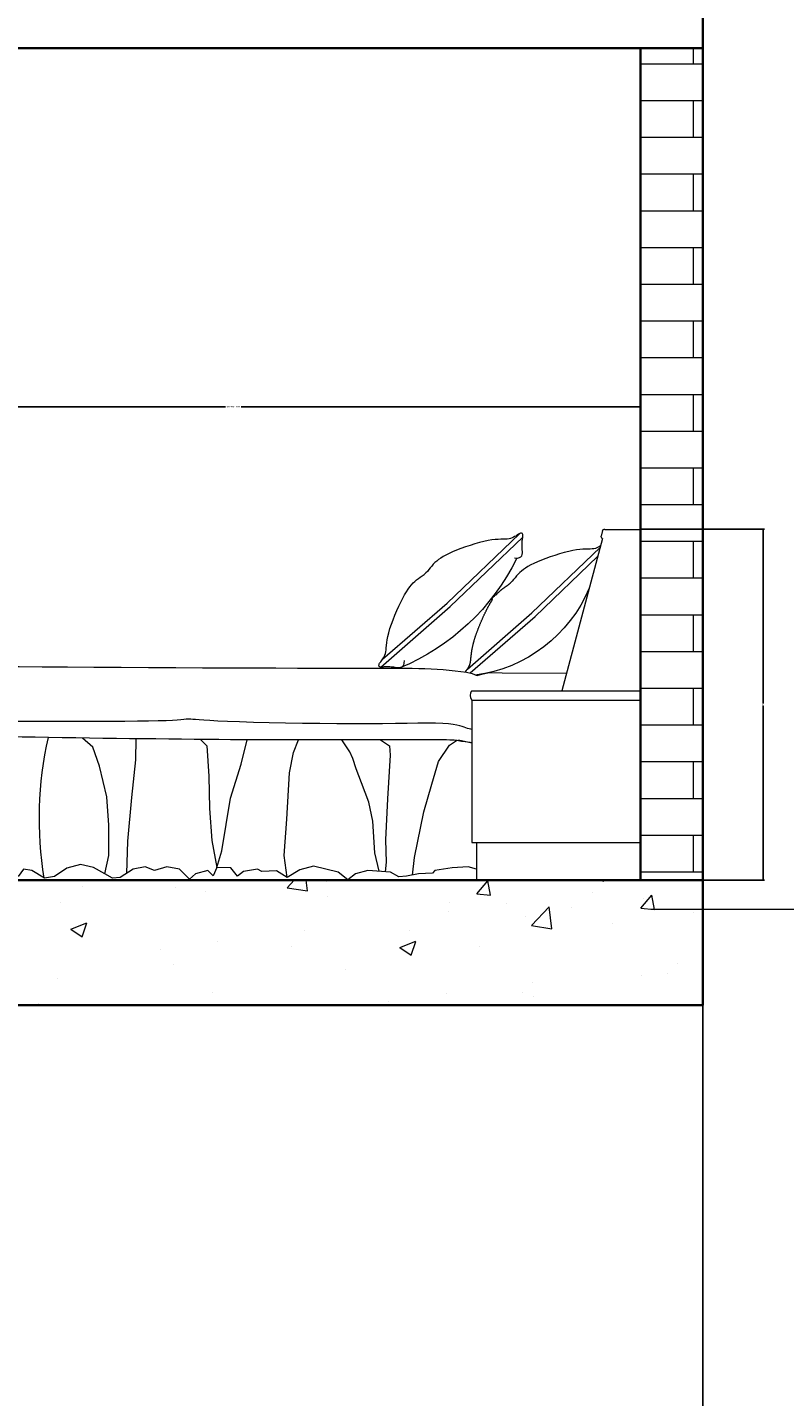
# Model space of a CAD drawing. Units: inches. Extents: x 2416 to 3391, y 1375 to 2496.
# Tile 11 of 13: x 3105 to 3215, y 2069 to 2267. Entities that reach past the tile are written whole.
import ezdxf

# ---------------------------------------------------------------- set-up
doc = ezdxf.new("R2010")
doc.units = ezdxf.units.IN
for name, color, linetype, lineweight in [('A-ANNO-DIMS', 2, 'Continuous', 18), ('A-ANNO-TEXT', 7, 'Continuous', 18), ('A-FLOR-PATT', 252, 'Continuous', 13), ('A-FURN', 8, 'Continuous', 18), ('A-SECT', 7, 'Continuous', 35), ('A-WALL-PATT', 252, 'Continuous', 13)]:
    doc.layers.add(name, color=color, linetype=linetype, lineweight=lineweight)
doc.styles.get("Standard").update_dxf_attribs({"font": 'arial.ttf'})
doc.dimstyles.get("Standard").update_dxf_attribs({"dimtxt": 0.18, "dimasz": 0.18, "dimexe": 0.18, "dimexo": 0.0625, "dimgap": 0.09, "dimtad": 0, "dimtih": 1, "dimtoh": 1, "dimdec": 4, "dimzin": 0, "dimdsep": 46, "dimtxsty": 'Standard', "dimcen": 0.09, "dimadec": 0, "dimazin": 0, "dimtfac": 1, "dimtdec": 4, "dimtofl": 0, "dimtmove": 0, "dimatfit": 3, "dimfxl": 1, "dimtolj": 1, "dimtzin": 0, "dimarcsym": 0})

# ---------------------------------------------------------------- blocks, each defined once
blk = doc.blocks.new('A$C08BC4B9A')
for p, q in [((0, 924.5), (0.5, 925)), ((0, 0), (0, 924.5)), ((95, 925), (0.5, 925)), ((101.1, 921.9), (105, 907.4)), ((311.4, 909.3), (311.5, 910.8)), ((311.5, 907.6), (311.4, 909.3)), ((311.5, 910.8), (311.7, 912.1)), ((311.7, 905.6), (311.5, 907.6)), ((311.7, 912.1), (312.1, 913.2)), ((312, 903.5), (311.7, 905.6)), ((502.9, 721.7), (311.9, 904.5)), ((312.3, 901.1), (312, 903.5)), ((312.1, 913.2), (312.7, 914.1)), ((312.7, 914.1), (313.6, 914.7)), ((313.6, 914.7), (314.7, 915)), ((314.7, 915), (316, 915.1)), ((316, 915.1), (317.6, 914.9)), ((317.6, 914.9), (319.3, 914.5)), ((319.3, 914.5), (321.1, 913.7)), ((511.6, 731.1), (320.5, 913.9)), ((321.1, 913.7), (323.2, 912.6)), ((323.2, 912.6), (325.4, 911.2)), ((325.4, 911.2), (327.8, 909.6)), ((327.8, 909.6), (330.4, 907.8)), ((330.4, 907.8), (333.3, 906.1)), ((333.3, 906.1), (336.4, 904.3)), ((336.4, 904.3), (339.9, 902.7)), ((339.9, 902.7), (343.7, 901.4)), ((101.4, 901.2), (208.9, 500)), ((106.6, 881.7), (106.8, 881.6)), ((106.8, 881.6), (109.7, 879.8)), ((288, 704.9), (107.8, 877.3)), ((109.7, 879.8), (112.8, 878.1)), ((112.8, 878.1), (116.3, 876.5)), ((116.3, 876.5), (120.1, 875.2)), ((120.1, 875.2), (124.3, 874.2)), ((124.3, 874.2), (128.9, 873.6)), ((128.9, 873.6), (134, 873.3)), ((134, 873.3), (139.6, 873.2)), ((139.6, 873.2), (146, 873)), ((146, 873), (153.1, 872.7)), ((153.1, 872.7), (161, 872.1)), ((161, 872.1), (169.8, 871.1)), ((169.8, 871.1), (179.7, 869.5)), ((179.7, 869.5), (190.6, 867.1)), ((190.6, 867.1), (202.3, 864.2)), ((312.6, 898.6), (312.3, 901.1)), ((312.9, 895.9), (312.6, 898.6)), ((312.7, 863.2), (312.8, 867.3)), ((312.8, 867.3), (313, 871.5)), ((313.1, 892.9), (312.9, 895.9)), ((313, 871.5), (313.3, 875.5)), ((313.3, 889.8), (313.1, 892.9)), ((313.4, 886.5), (313.3, 889.8)), ((313.3, 875.5), (313.4, 879.4)), ((313.4, 883), (313.4, 886.5)), ((313.4, 879.4), (313.4, 883)), ((343.7, 901.4), (347.9, 900.4)), ((347.9, 900.4), (352.5, 899.8)), ((352.5, 899.8), (357.6, 899.5)), ((357.6, 899.5), (363.2, 899.4)), ((363.2, 899.4), (369.6, 899.2)), ((369.6, 899.2), (376.7, 898.9)), ((376.7, 898.9), (384.6, 898.3)), ((384.6, 898.3), (393.4, 897.3)), ((393.4, 897.3), (403.3, 895.7)), ((403.3, 895.7), (414.2, 893.3)), ((414.2, 893.3), (425.9, 890.4)), ((425.9, 890.4), (438.1, 886.9)), ((438.1, 886.9), (450.5, 883.1)), ((450.5, 883.1), (462.9, 878.9)), ((462.9, 878.9), (474.9, 874.6)), ((474.9, 874.6), (486.3, 870.2)), ((486.3, 870.2), (496.8, 865.9)), ((279.2, 695.5), (114.2, 853.4)), ((202.3, 864.2), (214.5, 860.7)), ((214.5, 860.7), (226.9, 856.8)), ((226.9, 856.8), (239.3, 852.7)), ((239.3, 852.7), (251.3, 848.4)), ((251.3, 848.4), (262.7, 844)), ((262.7, 844), (273.2, 839.6)), ((273.2, 839.6), (282.5, 835.5)), ((282.5, 835.5), (290.7, 831.4)), ((290.7, 831.4), (298, 827.4)), ((313.1, 859.2), (312.7, 863.2)), ((314.3, 855.7), (313.1, 859.2)), ((316.7, 852.8), (314.3, 855.7)), ((320.4, 850.8), (316.7, 852.8)), ((325.8, 849.7), (320.4, 850.8)), ((333.2, 849.9), (325.8, 849.7)), ((496.8, 865.9), (506.1, 861.7)), ((506.1, 861.7), (514.3, 857.6)), ((514.3, 857.6), (521.6, 853.6)), ((521.6, 853.6), (528, 849.7)), ((528, 849.7), (533.7, 845.7)), ((533.7, 845.7), (538.8, 841.7)), ((538.8, 841.7), (543.4, 837.5)), ((543.4, 837.5), (547.7, 833.2)), ((547.7, 833.2), (551.7, 828.7)), ((298, 827.4), (304.4, 823.4)), ((304.4, 823.4), (310.1, 819.5)), ((310.1, 819.5), (315.2, 815.4)), ((315.2, 815.4), (319.8, 811.3)), ((319.8, 811.3), (324.1, 807)), ((324.1, 807), (328.1, 802.5)), ((328.1, 802.5), (332, 797.9)), ((332, 797.9), (335.8, 793.2)), ((551.7, 828.7), (555.6, 824.1)), ((555.6, 824.1), (559.4, 819.4)), ((559.4, 819.4), (563.3, 814.6)), ((563.3, 814.6), (567.7, 810.4)), ((572.2, 806.3), (567.7, 810.4)), ((577.3, 802.8), (572.2, 806.3)), ((582.3, 799.4), (577.3, 802.8)), ((587.2, 795.8), (582.3, 799.4)), ((592, 792.2), (587.2, 795.8)), ((335.8, 793.2), (339.7, 788.4)), ((339.7, 788.4), (344.1, 784.1)), ((344.2, 784), (344.1, 784.1)), ((344.5, 783.8), (344.2, 784)), ((344.9, 783.4), (344.5, 783.8)), ((345.5, 782.9), (344.9, 783.4)), ((346.1, 782.3), (345.5, 782.9)), ((346.8, 781.7), (346.1, 782.3)), ((347.6, 781.1), (346.8, 781.7)), ((348.3, 780.5), (347.6, 781.1)), ((349.1, 779.9), (348.3, 780.5)), ((349.8, 779.4), (349.1, 779.9)), ((350.5, 778.9), (349.8, 779.4)), ((351.1, 778.4), (350.5, 778.9)), ((351.8, 777.9), (351.1, 778.4)), ((352.4, 777.5), (351.8, 777.9)), ((353.1, 777), (352.4, 777.5)), ((353.7, 776.6), (353.1, 777)), ((354.3, 776.2), (353.7, 776.6)), ((354.9, 775.7), (354.3, 776.2)), ((355.6, 775.3), (354.9, 775.7)), ((356.2, 774.9), (355.6, 775.3)), ((356.8, 774.4), (356.2, 774.9)), ((357.4, 774), (356.8, 774.4)), ((358.1, 773.6), (357.4, 774)), ((358.7, 773.1), (358.1, 773.6)), ((359.3, 772.7), (358.7, 773.1)), ((359.9, 772.3), (359.3, 772.7)), ((360.5, 771.8), (359.9, 772.3)), ((361.2, 771.4), (360.5, 771.8)), ((361.8, 770.9), (361.2, 771.4)), ((362.4, 770.5), (361.8, 770.9)), ((363, 770), (362.4, 770.5)), ((363.6, 769.6), (363, 770)), ((364.2, 769.1), (363.6, 769.6)), ((364.8, 768.7), (364.2, 769.1)), ((365.4, 768.2), (364.8, 768.7)), ((366, 767.8), (365.4, 768.2)), ((366.6, 767.3), (366, 767.8)), ((367.2, 766.8), (366.6, 767.3)), ((367.8, 766.4), (367.2, 766.8)), ((368.3, 765.9), (367.8, 766.4)), ((368.9, 765.4), (368.3, 765.9)), ((369.5, 764.9), (368.9, 765.4)), ((370.1, 764.4), (369.5, 764.9)), ((370.7, 763.9), (370.1, 764.4)), ((371.2, 763.5), (370.7, 763.9)), ((371.8, 763), (371.2, 763.5)), ((372.4, 762.4), (371.8, 763)), ((373, 761.9), (372.4, 762.4)), ((373.5, 761.4), (373, 761.9)), ((374.1, 760.9), (373.5, 761.4)), ((374.7, 760.4), (374.1, 760.9)), ((375.2, 759.8), (374.7, 760.4)), ((375.8, 759.3), (375.2, 759.8)), ((376.3, 758.7), (375.8, 759.3)), ((376.9, 758.2), (376.3, 758.7)), ((377.4, 757.6), (376.9, 758.2)), ((596.6, 788.2), (592, 792.2)), ((601.1, 783.9), (596.6, 788.2)), ((605.5, 779.1), (601.1, 783.9)), ((609.9, 773.7), (605.5, 779.1)), ((614.3, 767.6), (609.9, 773.7)), ((618.8, 760.7), (614.3, 767.6)), ((623.5, 752.8), (618.8, 760.7)), ((378, 757), (377.4, 757.6)), ((378.6, 756.5), (378, 757)), ((379.2, 755.8), (378.6, 756.5)), ((379.8, 755.2), (379.2, 755.8)), ((380.5, 754.5), (379.8, 755.2)), ((381.3, 753.8), (380.5, 754.5)), ((382.2, 753.1), (381.3, 753.8)), ((383.2, 752.3), (382.2, 753.1)), ((384.2, 751.4), (383.2, 752.3)), ((385.4, 750.5), (384.2, 751.4)), ((386.6, 749.6), (385.4, 750.5)), ((387.8, 748.7), (386.6, 749.6)), ((388.9, 747.8), (387.8, 748.7)), ((389.9, 746.9), (388.9, 747.8)), ((390.8, 746), (389.9, 746.9)), ((391.4, 745.3), (390.8, 746)), ((391.9, 744.6), (391.4, 745.3)), ((392.1, 744), (391.9, 744.6)), ((392, 741.9), (392.1, 742.4)), ((392, 741.3), (392, 741.9)), ((392, 740.8), (392, 741.3)), ((392.1, 740.1), (392, 740.8)), ((392.2, 743.4), (392.1, 744)), ((392.1, 742.4), (392.2, 742.9)), ((392.4, 739.4), (392.1, 740.1)), ((392.2, 742.9), (392.2, 743.4)), ((392.7, 738.6), (392.4, 739.4)), ((393.1, 737.8), (392.7, 738.6)), ((393.6, 737), (393.1, 737.8)), ((394.1, 736.1), (393.6, 737)), ((394.7, 735.2), (394.1, 736.1)), ((395.2, 734.3), (394.7, 735.2)), ((395.8, 733.4), (395.2, 734.3)), ((396.4, 732.4), (395.8, 733.4)), ((397, 731.5), (396.4, 732.4)), ((397.6, 730.5), (397, 731.5)), ((398.2, 729.5), (397.6, 730.5)), ((398.7, 728.5), (398.2, 729.5)), ((399.3, 727.4), (398.7, 728.5)), ((399.9, 726.4), (399.3, 727.4)), ((400.5, 725.3), (399.9, 726.4)), ((401.1, 724.3), (400.5, 725.3)), ((401.7, 723.2), (401.1, 724.3)), ((402.4, 722), (401.7, 723.2)), ((681.3, 583.2), (511.6, 731.1)), ((628.4, 743.8), (623.5, 752.8)), ((633.5, 733.7), (628.4, 743.8)), ((638.7, 722.7), (633.5, 733.7)), ((643.9, 711), (638.7, 722.7)), ((450.1, 546.6), (279.2, 695.5)), ((457.7, 557), (288, 704.9)), ((403, 720.9), (402.4, 722)), ((403.6, 719.8), (403, 720.9)), ((404.2, 718.6), (403.6, 719.8)), ((404.8, 717.4), (404.2, 718.6)), ((405.4, 716.2), (404.8, 717.4)), ((406.1, 715), (405.4, 716.2)), ((406.7, 713.8), (406.1, 715)), ((407.3, 712.5), (406.7, 713.8)), ((408, 711.2), (407.3, 712.5)), ((408.6, 710), (408, 711.2)), ((409.3, 708.7), (408.6, 710)), ((409.9, 707.3), (409.3, 708.7)), ((410.6, 706), (409.9, 707.3)), ((411.2, 704.7), (410.6, 706)), ((411.9, 703.3), (411.2, 704.7)), ((412.5, 701.9), (411.9, 703.3)), ((413.2, 700.6), (412.5, 701.9)), ((413.8, 699.2), (413.2, 700.6)), ((414.5, 697.8), (413.8, 699.2)), ((415.1, 696.4), (414.5, 697.8)), ((415.8, 694.9), (415.1, 696.4)), ((416.4, 693.5), (415.8, 694.9)), ((417.1, 692.1), (416.4, 693.5)), ((417.7, 690.6), (417.1, 692.1)), ((418.4, 689.2), (417.7, 690.6)), ((419, 687.7), (418.4, 689.2)), ((419.7, 686.2), (419, 687.7)), ((420.3, 684.7), (419.7, 686.2)), ((685.7, 562.3), (502.9, 721.7)), ((649, 699), (643.9, 711)), ((653.8, 686.9), (649, 699)), ((658.2, 675), (653.8, 686.9)), ((421, 683.3), (420.3, 684.7)), ((421.6, 681.8), (421, 683.3)), ((422.2, 680.3), (421.6, 681.8)), ((422.9, 678.8), (422.2, 680.3)), ((423.5, 677.3), (422.9, 678.8)), ((424.1, 675.8), (423.5, 677.3)), ((424.7, 674.3), (424.1, 675.8)), ((425.4, 672.8), (424.7, 674.3)), ((426, 671.3), (425.4, 672.8)), ((426.6, 669.7), (426, 671.3)), ((427.2, 668.2), (426.6, 669.7)), ((427.8, 666.7), (427.2, 668.2)), ((428.4, 665.2), (427.8, 666.7)), ((429, 663.7), (428.4, 665.2)), ((429.6, 662.2), (429, 663.7)), ((430.1, 660.7), (429.6, 662.2)), ((430.7, 659.2), (430.1, 660.7)), ((431.3, 657.7), (430.7, 659.2)), ((431.8, 656.2), (431.3, 657.7)), ((432.4, 654.7), (431.8, 656.2)), ((432.9, 653.2), (432.4, 654.7)), ((433.4, 651.8), (432.9, 653.2)), ((434, 650.3), (433.4, 651.8)), ((434.5, 648.8), (434, 650.3)), ((662, 663.6), (658.2, 675)), ((665.2, 652.9), (662, 663.6)), ((667.5, 643.2), (665.2, 652.9)), ((435, 647.4), (434.5, 648.8)), ((435.5, 645.9), (435, 647.4)), ((436, 644.5), (435.5, 645.9)), ((436.5, 643.1), (436, 644.5)), ((436.9, 641.7), (436.5, 643.1)), ((437.4, 640.2), (436.9, 641.7)), ((437.9, 638.8), (437.4, 640.2)), ((438.3, 637.5), (437.9, 638.8)), ((438.7, 636.1), (438.3, 637.5)), ((439.1, 634.7), (438.7, 636.1)), ((439.6, 633.4), (439.1, 634.7)), ((440, 632), (439.6, 633.4)), ((440.3, 630.7), (440, 632)), ((440.7, 629.4), (440.3, 630.7)), ((441.1, 628.1), (440.7, 629.4)), ((441.4, 626.8), (441.1, 628.1)), ((441.8, 625.5), (441.4, 626.8)), ((442.1, 624.3), (441.8, 625.5)), ((442.4, 623.1), (442.1, 624.3)), ((442.7, 621.8), (442.4, 623.1)), ((443, 620.6), (442.7, 621.8)), ((443.3, 619.4), (443, 620.6)), ((443.6, 618.3), (443.3, 619.4)), ((443.8, 617.1), (443.6, 618.3)), ((444.1, 616), (443.8, 617.1)), ((444.3, 614.8), (444.1, 616)), ((444.5, 613.7), (444.3, 614.8)), ((669.2, 634.4), (667.5, 643.2)), ((670.4, 626.6), (669.2, 634.4)), ((671.3, 619.5), (670.4, 626.6)), ((671.9, 613.2), (671.3, 619.5)), ((444.7, 612.6), (444.5, 613.7)), ((445, 611.5), (444.7, 612.6)), ((445.2, 610.5), (445, 611.5)), ((445.4, 609.4), (445.2, 610.5)), ((445.5, 608.4), (445.4, 609.4)), ((445.7, 607.3), (445.5, 608.4)), ((445.9, 606.3), (445.7, 607.3)), ((446, 605.3), (445.9, 606.3)), ((446.2, 604.3), (446, 605.3)), ((446.4, 603.3), (446.2, 604.3)), ((446.5, 602.4), (446.4, 603.3)), ((446.6, 601.4), (446.5, 602.4)), ((446.8, 600.5), (446.6, 601.4)), ((446.9, 599.6), (446.8, 600.5)), ((447, 598.6), (446.9, 599.6)), ((447.1, 597.7), (447, 598.6)), ((447.2, 596.9), (447.1, 597.7)), ((447.3, 596), (447.2, 596.9)), ((447.4, 595.1), (447.3, 596)), ((447.5, 594.3), (447.4, 595.1)), ((447.6, 593.4), (447.5, 594.3)), ((447.7, 592.6), (447.6, 593.4)), ((447.8, 591.8), (447.7, 592.6)), ((447.9, 591), (447.8, 591.8)), ((448, 590.2), (447.9, 591)), ((448, 589.4), (448, 590.2)), ((448.1, 588.6), (448, 589.4)), ((448.2, 587.9), (448.1, 588.6)), ((448.3, 587.1), (448.2, 587.9)), ((448.3, 586.4), (448.3, 587.1)), ((448.4, 585.6), (448.3, 586.4)), ((448.5, 584.9), (448.4, 585.6)), ((448.6, 584.2), (448.5, 584.9)), ((448.6, 583.5), (448.6, 584.2)), ((448.7, 582.8), (448.6, 583.5)), ((448.8, 582.1), (448.7, 582.8)), ((448.9, 581.4), (448.8, 582.1)), ((448.9, 580.8), (448.9, 581.4)), ((449, 580.1), (448.9, 580.8)), ((449.1, 579.5), (449, 580.1)), ((449.2, 578.8), (449.1, 579.5)), ((449.3, 578.2), (449.2, 578.8)), ((449.4, 577.6), (449.3, 578.2)), ((624.8, 579.5), (625.2, 572.1)), ((672.5, 607.6), (671.9, 613.2)), ((673.1, 602.5), (672.5, 607.6)), ((674.1, 598), (673.1, 602.5)), ((675.4, 593.9), (674.1, 598)), ((677, 590.2), (675.4, 593.9)), ((678.8, 586.8), (677, 590.2)), ((680.8, 583.8), (678.8, 586.8)), ((682.8, 581.1), (680.8, 583.8)), ((684.7, 578.6), (682.8, 581.1)), ((686.5, 576.4), (684.7, 578.6)), ((366.1, 546.8), (196.6, 546.1)), ((400.7, 547.5), (366.1, 546.8)), ((420, 543.6), (400.7, 547.5)), ((431.7, 540.1), (420, 543.6)), ((439.4, 542.5), (431.7, 540.1)), ((445.4, 545.7), (439.4, 542.5)), ((460.2, 548.4), (445.4, 545.7)), ((449.5, 577), (449.4, 577.6)), ((449.6, 576.4), (449.5, 577)), ((449.7, 575.8), (449.6, 576.4)), ((449.8, 575.2), (449.7, 575.8)), ((449.9, 574.6), (449.8, 575.2)), ((450, 574), (449.9, 574.6)), ((450.1, 573.5), (450, 574)), ((450.3, 572.9), (450.1, 573.5)), ((450.4, 572.4), (450.3, 572.9)), ((450.5, 571.8), (450.4, 572.4)), ((450.7, 571.3), (450.5, 571.8)), ((450.8, 570.8), (450.7, 571.3)), ((451, 570.2), (450.8, 570.8)), ((451.1, 569.7), (451, 570.2)), ((451.3, 569.2), (451.1, 569.7)), ((451.5, 568.7), (451.3, 569.2)), ((451.6, 568.2), (451.5, 568.7)), ((451.8, 567.7), (451.6, 568.2)), ((452, 567.2), (451.8, 567.7)), ((452.2, 566.8), (452, 567.2)), ((452.4, 566.3), (452.2, 566.8)), ((452.6, 565.8), (452.4, 566.3)), ((452.8, 565.4), (452.6, 565.8)), ((453, 564.9), (452.8, 565.4)), ((453.2, 564.5), (453, 564.9)), ((453.4, 564), (453.2, 564.5)), ((453.6, 563.6), (453.4, 564)), ((453.8, 563.1), (453.6, 563.6)), ((454.1, 562.7), (453.8, 563.1)), ((454.3, 562.3), (454.1, 562.7)), ((454.5, 561.9), (454.3, 562.3)), ((454.8, 561.5), (454.5, 561.9)), ((455, 561.1), (454.8, 561.5)), ((455.2, 560.7), (455, 561.1)), ((455.5, 560.3), (455.2, 560.7)), ((455.7, 559.9), (455.5, 560.3)), ((456, 559.5), (455.7, 559.9)), ((456.2, 559.1), (456, 559.5)), ((456.4, 558.8), (456.2, 559.1)), ((456.7, 558.4), (456.4, 558.8)), ((456.9, 558), (456.7, 558.4)), ((457.2, 557.7), (456.9, 558)), ((457.4, 557.3), (457.2, 557.7)), ((457.7, 557), (457.4, 557.3)), ((457.9, 556.6), (457.7, 557)), ((458.2, 556.3), (457.9, 556.6)), ((458.4, 555.9), (458.2, 556.3)), ((458.7, 555.6), (458.4, 555.9)), ((458.9, 555.3), (458.7, 555.6)), ((459.2, 554.9), (458.9, 555.3)), ((459.4, 554.6), (459.2, 554.9)), ((459.7, 554.3), (459.4, 554.6)), ((459.9, 554), (459.7, 554.3)), ((460.2, 553.6), (459.9, 554)), ((460.4, 553.3), (460.2, 553.6)), ((475.2, 550.7), (460.2, 548.4)), ((460.7, 553), (460.4, 553.3)), ((461, 552.6), (460.7, 553)), ((461.3, 552.3), (461, 552.6)), ((461.6, 551.9), (461.3, 552.3)), ((461.9, 551.5), (461.6, 551.9)), ((462.2, 551.1), (461.9, 551.5)), ((462.5, 550.7), (462.2, 551.1)), ((462.8, 550.3), (462.5, 550.7)), ((463.2, 549.8), (462.8, 550.3)), ((463.5, 549.4), (463.2, 549.8)), ((463.8, 548.9), (463.5, 549.4)), ((490.5, 552.6), (475.2, 550.7)), ((506, 554.2), (490.5, 552.6)), ((521.7, 555.5), (506, 554.2)), ((537.6, 556.6), (521.7, 555.5)), ((553.6, 557.4), (537.6, 556.6)), ((569.7, 558.1), (553.6, 557.4)), ((586, 558.6), (569.7, 558.1)), ((603.2, 559), (586, 558.6)), ((621.8, 559.3), (603.2, 559)), ((642.6, 559.5), (621.8, 559.3)), ((625.2, 572.1), (626.6, 566.8)), ((626.6, 566.8), (629, 563.3)), ((629, 563.3), (632, 561.2)), ((632, 561.2), (635.6, 560.2)), ((635.6, 560.2), (639.6, 560.1)), ((639.6, 560.1), (643.7, 560.5)), ((666.5, 559.6), (642.6, 559.5)), ((643.7, 560.5), (647.9, 561)), ((647.9, 561), (651.9, 561.6)), ((651.9, 561.6), (655.7, 562)), ((655.7, 562), (659.3, 562.3)), ((659.3, 562.3), (662.8, 562.5)), ((662.8, 562.5), (666.1, 562.7)), ((666.1, 562.7), (669.2, 562.7)), ((693.9, 559.6), (666.5, 559.6)), ((669.2, 562.7), (672.2, 562.7)), ((672.2, 562.7), (674.9, 562.7)), ((674.9, 562.7), (677.5, 562.6)), ((677.5, 562.6), (679.8, 562.4)), ((679.8, 562.4), (682, 562.3)), ((682, 562.3), (683.9, 562.3)), ((683.9, 562.3), (685.7, 562.3)), ((685.7, 562.3), (687.2, 562.4)), ((688.1, 574.3), (686.5, 576.4)), ((687.2, 562.4), (688.5, 562.7)), ((689.3, 572.3), (688.1, 574.3)), ((688.5, 562.7), (689.5, 563.2)), ((690.2, 570.5), (689.3, 572.3)), ((689.5, 563.2), (690.3, 563.9)), ((690.8, 568.8), (690.2, 570.5)), ((690.3, 563.9), (690.9, 564.9)), ((691.1, 567.3), (690.8, 568.8)), ((690.9, 564.9), (691.1, 566)), ((691.1, 566), (691.1, 567.3)), ((725.8, 559.7), (693.9, 559.6)), ((762.8, 559.7), (725.8, 559.7)), ((805.4, 559.7), (762.8, 559.7)), ((853.4, 559.7), (805.4, 559.7)), ((906.2, 559.7), (853.4, 559.7)), ((963.4, 559.8), (906.2, 559.7)), ((1024.6, 559.9), (963.4, 559.8)), ((1089.2, 560.1), (1024.6, 559.9)), ((1156.7, 560.4), (1089.2, 560.1)), ((1226.8, 560.7), (1156.7, 560.4)), ((1298.7, 561.1), (1226.8, 560.7)), ((1371.2, 561.6), (1298.7, 561.1)), ((1443.1, 562.1), (1371.2, 561.6)), ((1512.8, 562.6), (1443.1, 562.1)), ((1579.1, 563), (1512.8, 562.6)), ((1640.5, 563.3), (1579.1, 563)), ((1695.8, 563.4), (1640.5, 563.3)), ((1743.5, 563.3), (1695.8, 563.4)), ((1782.8, 563), (1743.5, 563.3)), ((1814.2, 562.4), (1782.8, 563)), ((1838.9, 561.5), (1814.2, 562.4)), ((1858, 560.2), (1838.9, 561.5)), ((1872.6, 558.6), (1858, 560.2)), ((1883.7, 556.6), (1872.6, 558.6)), ((1892.6, 554.2), (1883.7, 556.6)), ((1900.3, 551.3), (1892.6, 554.2)), ((1907.7, 547.9), (1900.3, 551.3)), ((1915, 544), (1907.7, 547.9)), ((1922.1, 539.6), (1915, 544)), ((1929, 534.5), (1922.1, 539.6)), ((1935.8, 528.9), (1929, 534.5)), ((1942.3, 522.6), (1935.8, 528.9)), ((1948.6, 515.6), (1942.3, 522.6)), ((1954.6, 508), (1948.6, 515.6)), ((1960.4, 499.6), (1954.6, 508)), ((445.9, 500), (0, 500)), ((445.9, 475), (0, 475)), ((445.9, 475), (445.9, 100)), ((1965.8, 490.7), (1960.4, 499.6)), ((1970.9, 481.5), (1965.8, 490.7)), ((1975.6, 472.1), (1970.9, 481.5)), ((1980, 462.7), (1975.6, 472.1)), ((1984, 453.6), (1980, 462.7)), ((1987.5, 445), (1984, 453.6)), ((1990.7, 437), (1987.5, 445)), ((1993.4, 429.7), (1990.7, 437)), ((445.9, 397.8), (449.1, 398.3)), ((449.1, 398.3), (453.4, 399.2)), ((453.4, 399.2), (457.6, 400.4)), ((457.6, 400.4), (461.8, 402)), ((461.8, 402), (466.2, 403.7)), ((466.2, 403.7), (471.3, 405.6)), ((471.3, 405.6), (477.6, 407.5)), ((477.6, 407.5), (485.4, 409.4)), ((485.4, 409.4), (495.3, 411.1)), ((495.3, 411.1), (507.7, 412.5)), ((507.7, 412.5), (523, 413.5)), ((523, 413.5), (541.5, 414)), ((541.5, 414), (563.2, 414.2)), ((563.2, 414.2), (588.2, 414.1)), ((588.2, 414.1), (616.4, 413.7)), ((616.4, 413.7), (647.7, 413.3)), ((647.7, 413.3), (682, 412.9)), ((682, 412.9), (719.4, 412.6)), ((719.4, 412.6), (759.7, 412.4)), ((759.7, 412.4), (802.6, 412.6)), ((802.6, 412.6), (847.4, 413)), ((847.4, 413), (892.8, 413.6)), ((892.8, 413.6), (937.8, 414.4)), ((937.8, 414.4), (981.1, 415.3)), ((981.1, 415.3), (1021.7, 416.4)), ((1021.7, 416.4), (1058.6, 417.5)), ((1058.6, 417.5), (1090.4, 418.7)), ((1090.4, 418.7), (1116.5, 419.9)), ((1116.5, 419.9), (1137.2, 421)), ((1137.2, 421), (1153.4, 422.1)), ((1153.4, 422.1), (1165.7, 423)), ((1165.7, 423), (1174.9, 423.8)), ((1174.9, 423.8), (1181.7, 424.4)), ((1181.7, 424.4), (1186.9, 424.8)), ((1186.9, 424.8), (1191.2, 425)), ((1191.2, 425), (1195.4, 424.8)), ((1195.4, 424.8), (1200, 424.5)), ((1200, 424.5), (1205.8, 423.9)), ((1205.8, 423.9), (1213.3, 423.2)), ((1213.3, 423.2), (1223.1, 422.4)), ((1223.1, 422.4), (1236, 421.7)), ((1236, 421.7), (1252.5, 420.9)), ((1252.5, 420.9), (1273.3, 420.3)), ((1273.3, 420.3), (1298.7, 419.7)), ((1298.7, 419.7), (1328.3, 419.4)), ((1328.3, 419.4), (1361.1, 419.1)), ((1361.1, 419.1), (1396.4, 418.9)), ((1396.4, 418.9), (1433.4, 418.8)), ((1433.4, 418.8), (1471.3, 418.7)), ((1471.3, 418.7), (1509.3, 418.7)), ((1509.3, 418.7), (1546.6, 418.7)), ((1546.6, 418.7), (1582.4, 418.7)), ((1582.4, 418.7), (1616.7, 418.7)), ((1616.7, 418.7), (1649.3, 418.7)), ((1649.3, 418.7), (1680.1, 418.7)), ((1680.1, 418.7), (1709, 418.7)), ((1709, 418.7), (1736, 418.7)), ((1736, 418.7), (1760.9, 418.7)), ((1760.9, 418.7), (1783.8, 418.7)), ((1783.8, 418.7), (1804.5, 418.7)), ((1804.5, 418.7), (1823.2, 418.6)), ((1823.2, 418.6), (1840.3, 418.5)), ((1840.3, 418.5), (1856.1, 418.1)), ((1856.1, 418.1), (1870.7, 417.6)), ((1870.7, 417.6), (1884.5, 416.7)), ((1884.5, 416.7), (1897.8, 415.6)), ((1897.8, 415.6), (1910.8, 414)), ((1910.8, 414), (1923.7, 412)), ((1923.7, 412), (1936.5, 409.7)), ((1936.5, 409.7), (1949.1, 407.1)), ((1949.1, 407.1), (1961.3, 404.4)), ((1961.3, 404.4), (1973.1, 401.6)), ((1973.1, 401.6), (1984.4, 398.8)), ((1984.4, 398.8), (1995, 396.1)), ((1995.8, 423.3), (1993.4, 429.7)), ((1997.8, 417.5), (1995.8, 423.3)), ((1999.6, 412.4), (1997.8, 417.5)), ((2001.3, 407.8), (1999.6, 412.4)), ((2002.8, 403.7), (2001.3, 407.8)), ((2004.3, 400.1), (2002.8, 403.7)), ((2005.8, 396.8), (2004.3, 400.1)), ((445.9, 362), (481.5, 369.7)), ((445.9, 362.5), (450.4, 363.2)), ((450.4, 363.2), (457.2, 364.1)), ((457.2, 364.1), (463.4, 364.9)), ((463.4, 364.9), (468.9, 365.7)), ((468.9, 365.7), (473.6, 366.4)), ((473.6, 366.4), (477.6, 367.1)), ((477.6, 367.1), (481.1, 367.7)), ((481.1, 367.7), (484.4, 368.3)), ((484.4, 368.3), (488, 368.8)), ((504.7, 356.4), (486.2, 368.5)), ((488, 368.8), (492.3, 369.2)), ((492.3, 369.2), (497.5, 369.6)), ((497.5, 369.6), (504.1, 369.9)), ((504.1, 369.9), (512.5, 370.1)), ((512.5, 370.1), (522.9, 370.3)), ((522.9, 370.3), (535.3, 370.3)), ((535.3, 370.3), (549.5, 370.3)), ((549.5, 370.3), (565.4, 370.3)), ((565.4, 370.3), (582.8, 370.2)), ((582.8, 370.2), (601.6, 370.2)), ((601.6, 370.2), (621.6, 370.1)), ((621.6, 370.1), (642.7, 370.1)), ((642.7, 370.1), (664.7, 370.1)), ((687.3, 370.2), (663.6, 354.7)), ((664.7, 370.1), (687.3, 370.2)), ((687.3, 370.2), (710.4, 370.3)), ((710.4, 370.3), (733.4, 370.4)), ((733.4, 370.4), (756.3, 370.4)), ((756.3, 370.4), (778.7, 370.5)), ((768.3, 339), (789.4, 370.5)), ((778.7, 370.5), (800.2, 370.6)), ((800.2, 370.6), (820.7, 370.6)), ((820.7, 370.6), (840, 370.6)), ((840, 370.6), (858.3, 370.5)), ((858.3, 370.5), (876.2, 370.4)), ((876.2, 370.4), (894, 370.4)), ((894, 370.4), (912.3, 370.3)), ((916.7, 337.2), (903.2, 370.3)), ((912.3, 370.3), (931.5, 370.2)), ((931.5, 370.2), (952, 370.2)), ((952, 370.2), (974.3, 370.2)), ((974.3, 370.2), (998.7, 370.3)), ((998.7, 370.3), (1025.1, 370.4)), ((1025.1, 370.4), (1053.2, 370.6)), ((1054.7, 305.8), (1039.1, 370.5)), ((1053.2, 370.6), (1082.9, 370.8)), ((1082.9, 370.8), (1113.8, 371)), ((1113.8, 371), (1145.8, 371.3)), ((1162.2, 371.4), (1145.5, 354.7)), ((1145.8, 371.3), (1178.6, 371.6)), ((1178.6, 371.6), (1212, 371.9)), ((1212, 371.9), (1245.7, 372.2)), ((1245.7, 372.2), (1279.8, 372.6)), ((1279.8, 372.6), (1314.1, 373)), ((1314.1, 373), (1348.8, 373.4)), ((1332.3, 318), (1331.5, 373.2)), ((1348.8, 373.4), (1383.8, 373.8)), ((1383.8, 373.8), (1419.1, 374.3)), ((1419.1, 374.3), (1454.7, 374.8)), ((1445.8, 351.2), (1472.7, 375.1)), ((1454.7, 374.8), (1490.6, 375.4)), ((1490.6, 375.4), (1526.8, 376)), ((1526.8, 376), (1562.7, 376.6)), ((1562.7, 376.6), (1597.9, 377.2)), ((1597.9, 377.2), (1632, 377.8)), ((1632, 377.8), (1664.4, 378.4)), ((1664.4, 378.4), (1694.6, 378.9)), ((1694.6, 378.9), (1722.2, 379.3)), ((1722.2, 379.3), (1746.7, 379.5)), ((1746.7, 379.5), (1767.7, 379.7)), ((1767.7, 379.7), (1785.7, 379.6)), ((1785.7, 379.6), (1801.2, 379.4)), ((1801.2, 379.4), (1814.9, 378.9)), ((1814.9, 378.9), (1827.4, 378.2)), ((1827.4, 378.2), (1839.2, 377.2)), ((1839.2, 377.2), (1850.9, 375.9)), ((1845.1, 376.6), (1887, 298.9)), ((1850.9, 375.9), (1863.2, 374.3)), ((1863.2, 374.3), (1876.4, 372.4)), ((1876.4, 372.4), (1890.5, 370.2)), ((1890.5, 370.2), (1905, 367.7)), ((1905, 367.7), (1919.7, 364.9)), ((1919.7, 364.9), (1934.2, 362)), ((1934.2, 362), (1948.2, 358.9)), ((1995, 396.1), (2004.8, 393.6)), ((2007.5, 393.8), (2005.8, 396.8)), ((2009.2, 390.9), (2007.5, 393.8)), ((2010.9, 388.2), (2009.2, 390.9)), ((2012.7, 385.4), (2010.9, 388.2)), ((2014.5, 382.5), (2012.7, 385.4)), ((2016.4, 379.3), (2014.5, 382.5)), ((2018.2, 375.7), (2016.4, 379.3)), ((2020, 371.7), (2018.2, 375.7)), ((2021.7, 367.2), (2020, 371.7)), ((2023.2, 362.2), (2021.7, 367.2)), ((2024.6, 357.2), (2023.2, 362.2)), ((534.3, 312.8), (504.7, 356.4)), ((663.6, 354.7), (661.8, 330.2)), ((661.8, 330.2), (668.8, 215.1)), ((759.6, 321.5), (768.3, 339)), ((927.2, 283.1), (916.7, 337.2)), ((1145.5, 354.7), (1140.2, 274.4)), ((1428.3, 300.6), (1445.8, 351.2)), ((1948.2, 358.9), (1961.4, 355.7)), ((1961.4, 355.7), (1973.5, 352.4)), ((1973.5, 352.4), (1984.1, 349.1)), ((1977.1, 352.6), (1976.8, 353.5)), ((1978, 350), (1977.1, 352.6)), ((1979.4, 346.1), (1978, 350)), ((1981.2, 341.1), (1979.4, 346.1)), ((1983.2, 335.3), (1981.2, 341.1)), ((1985.5, 329), (1983.2, 335.3)), ((1984.1, 349.1), (1993.3, 345.9)), ((1987.8, 322.5), (1985.5, 329)), ((1993.3, 345.9), (2001.3, 342.9)), ((2001.3, 342.9), (2007.9, 340.5)), ((2007.9, 340.5), (2013.4, 338.6)), ((2013.4, 338.6), (2017.8, 337.5)), ((2015, 211.3), (2015, 338.2)), ((2017.8, 337.5), (2021.2, 337.3)), ((2021.2, 337.3), (2023.6, 338.3)), ((2023.6, 338.3), (2025.2, 340.5)), ((2025.5, 352.3), (2024.6, 357.2)), ((2025.2, 340.5), (2025.9, 343.7)), ((2026, 347.7), (2025.5, 352.3)), ((2025.9, 343.7), (2026, 347.7)), ((551.8, 253.5), (534.3, 312.8)), ((736.9, 257), (750.9, 293.6)), ((750.9, 293.6), (759.6, 321.5)), ((1082.6, 216.8), (1054.7, 305.8)), ((1342.8, 218.6), (1332.3, 318)), ((1409.1, 220.3), (1428.3, 300.6)), ((1887, 298.9), (1932.4, 164.5)), ((1990.1, 316.1), (1987.8, 322.5)), ((1992.3, 309.9), (1990.1, 316.1)), ((1994.4, 304), (1992.3, 309.9)), ((1996.4, 298.3), (1994.4, 304)), ((1998.2, 292.7), (1996.4, 298.3)), ((2000, 287.1), (1998.2, 292.7)), ((572.8, 180.2), (551.8, 253.5)), ((717.7, 206.4), (736.9, 257)), ((934.2, 161), (927.2, 283.1)), ((1140.2, 274.4), (1138.5, 188.9)), ((2001.6, 281.3), (2000, 287.1)), ((2003.1, 275.4), (2001.6, 281.3)), ((2004.5, 269.2), (2003.1, 275.4)), ((2005.8, 262.6), (2004.5, 269.2)), ((2006.9, 255.8), (2005.8, 262.6)), ((2008, 248.9), (2006.9, 255.8)), ((1105.3, 77.3), (1082.6, 216.8)), ((1353.2, 103.4), (1342.8, 218.6)), ((1403.9, 145.3), (1409.1, 220.3)), ((2009, 242.1), (2008, 248.9)), ((2010, 235.6), (2009, 242.1)), ((2011, 229.5), (2010, 235.6)), ((2011.9, 223.9), (2011, 229.5)), ((2012.9, 219), (2011.9, 223.9)), ((2013.9, 215), (2012.9, 219)), ((668.8, 215.1), (674, 106.9)), ((707.2, 155.8), (717.7, 206.4)), ((1138.5, 188.9), (1131.5, 105.2)), ((2014.9, 211.6), (2013.9, 215)), ((2015.9, 208.7), (2014.9, 211.6)), ((2017, 206), (2015.9, 208.7)), ((2018.1, 203.5), (2017, 206)), ((2019.2, 200.8), (2018.1, 203.5)), ((2020.3, 197.8), (2019.2, 200.8)), ((2021.4, 194.3), (2020.3, 197.8)), ((2022.5, 190.2), (2021.4, 194.3)), ((2023.7, 185.5), (2022.5, 190.2)), ((2024.9, 180.4), (2023.7, 185.5)), ((597.2, 59.8), (572.8, 180.2)), ((702, 72), (707.2, 155.8)), ((941.2, 65.1), (934.2, 161)), ((1403.9, 65.1), (1403.9, 145.3)), ((1932.4, 164.5), (1951.6, 66.8)), ((2026.1, 175.1), (2024.9, 180.4)), ((2027.4, 169.8), (2026.1, 175.1)), ((2028.9, 164.7), (2027.4, 169.8)), ((2030.5, 159.8), (2028.9, 164.7)), ((2032.2, 155.5), (2030.5, 159.8)), ((2034.1, 151.8), (2032.2, 155.5)), ((2036.1, 148.6), (2034.1, 151.8)), ((2038.3, 145.9), (2036.1, 148.6)), ((2040.5, 143.6), (2038.3, 145.9)), ((2042.8, 141.5), (2040.5, 143.6)), ((2045, 139.6), (2042.8, 141.5)), ((2047.3, 137.8), (2045, 139.6)), ((2049.5, 136), (2047.3, 137.8)), ((2051.6, 134.1), (2049.5, 136)), ((2053.6, 132), (2051.6, 134.1)), ((2055.6, 129.7), (2053.6, 132)), ((2057.4, 127.3), (2055.6, 129.7)), ((2059.1, 124.7), (2057.4, 127.3)), ((2060.8, 121.9), (2059.1, 124.7)), ((2062.3, 118.9), (2060.8, 121.9)), ((2063.8, 115.6), (2062.3, 118.9)), ((2065.1, 112), (2063.8, 115.6)), ((2066.4, 108.3), (2065.1, 112)), ((445.9, 100), (0, 100)), ((433.9, 100), (433.9, 0)), ((674, 106.9), (672.3, 47.6)), ((1119, 34), (1105.3, 77.3)), ((1131.5, 105.2), (1119, 34)), ((1356.3, 18.2), (1353.2, 103.4)), ((2067.5, 104.3), (2066.4, 108.3)), ((2068.6, 100.2), (2067.5, 104.3)), ((2069.5, 95.9), (2068.6, 100.2)), ((2070.4, 91.5), (2069.5, 95.9)), ((2071.2, 87), (2070.4, 91.5)), ((2072, 82.5), (2071.2, 87)), ((2072.6, 77.9), (2072, 82.5)), ((2073.3, 73.2), (2072.6, 77.9)), ((2073.9, 68.1), (2073.3, 73.2)), ((602.8, 13.7), (597.2, 59.8)), ((672.3, 47.6), (674.3, 22.6)), ((690.4, 23.9), (702, 72)), ((798.3, 21.5), (864, 37.2)), ((864, 37.2), (900, 27.8)), ((932.8, 7.5), (941.2, 65.1)), ((1414.2, 16.7), (1403.9, 65.1)), ((1443.9, 33.9), (1478.3, 41.7)), ((1478.3, 41.7), (1514.3, 32.3)), ((1867.9, 15.1), (1897.6, 37)), ((1897.6, 37), (1928.9, 47.9)), ((1928.9, 47.9), (1968, 41.7)), ((1951.6, 66.8), (1948.4, 44.8)), ((1968, 41.7), (1980.5, 21.4)), ((1991.4, 8.9), (2014.9, 40.1)), ((2014.9, 40.1), (2044.6, 47.9)), ((2044.6, 47.9), (2079, 30.7)), ((2074.7, 62.4), (2073.9, 68.1)), ((2075.5, 56), (2074.7, 62.4)), ((2076.5, 48.7), (2075.5, 56)), ((2077.6, 40.3), (2076.5, 48.7)), ((2079, 30.7), (2077.6, 40.3)), ((0, 0), (2150.5, 0)), ((433.9, 29.5), (455.7, 35.6)), ((455.7, 35.6), (497.9, 32.5)), ((497.9, 32.5), (543.3, 26.2)), ((543.3, 26.2), (549.6, 18.4)), ((549.6, 18.4), (587.1, 16.9)), ((587.1, 16.9), (618.4, 10.6)), ((618.4, 10.6), (638.7, 9)), ((638.7, 9), (660.6, 21.5)), ((660.6, 21.5), (720.1, 26.2)), ((720.1, 26.2), (752.9, 16.9)), ((752.9, 16.9), (773.3, 1.2)), ((773.3, 1.2), (798.3, 21.5)), ((900, 27.8), (932.8, 7.5)), ((932.8, 7.5), (961, 24.7)), ((961, 24.7), (1000.1, 23.1)), ((1000.1, 23.1), (1011.1, 29.4)), ((1011.1, 29.4), (1048.6, 23.1)), ((1048.6, 23.1), (1064.3, 10.6)), ((1064.3, 10.6), (1081.5, 32.5)), ((1081.5, 32.5), (1119, 34)), ((1119, 34), (1128.4, 12.2)), ((1128.4, 12.2), (1142.5, 26.2)), ((1142.5, 26.2), (1175.3, 16.9)), ((1175.3, 16.9), (1191, 2.8)), ((1191, 2.8), (1217.6, 29.4)), ((1217.6, 29.4), (1250.4, 35.6)), ((1250.4, 35.6), (1283.3, 26.2)), ((1283.3, 26.2), (1307.8, 35.4)), ((1307.8, 35.4), (1339.1, 29.2)), ((1339.1, 29.2), (1373.5, 7.3)), ((1373.5, 7.3), (1393.8, 5.7)), ((1393.8, 5.7), (1414.2, 16.7)), ((1414.2, 16.7), (1443.9, 33.9)), ((1514.3, 32.3), (1547.2, 10.4)), ((1547.2, 10.4), (1573.7, 5.7)), ((1573.7, 5.7), (1606.6, 26.1)), ((1606.6, 26.1), (1628.5, 29.2)), ((1628.5, 29.2), (1642.6, 10.4)), ((1642.6, 10.4), (1667.6, 24.5)), ((1667.6, 24.5), (1705.2, 16.7)), ((1705.2, 16.7), (1714.5, 18.2)), ((1714.5, 18.2), (1730.2, 27.6)), ((1730.2, 27.6), (1745.8, 27.6)), ((1745.8, 27.6), (1753.7, 27.6)), ((1753.7, 27.6), (1786.5, 30.7)), ((1786.5, 30.7), (1799, 24.5)), ((1799, 24.5), (1814.7, 8.9)), ((1814.7, 8.9), (1867.9, 15.1)), ((1980.5, 21.4), (1991.4, 8.9)), ((2079, 30.7), (2095.6, 0))]:
    blk.add_line(p, q)
for centre, radius, start, end in [((96.2, 920.6), 5, 15, 105), ((100.1, 906.1), 5, 285, 15), ((863.9, 1112.1), 597.2, 206.2473, 247.5264), ((487.1, 917.9), 380.4, 202.7795, 262.4477), ((429, 487.5), 21, 323.3696, 36.6304), ((634, 163.3), 952.9, 350.4806, 12.9339), ((2353.4, 135.1), 676.8, 158.8487, 189.7401), ((6455, -433.2), 4778, 170.2062, 172.8555), ((1887.2, 90.1), 187, 157.7155, 202.6016), ((2056.3, 0.1), 84.2, 359.9053, 78.7345)]:
    blk.add_arc(centre, radius, start, end)
blk = doc.blocks.new('*D45')
at = {"layer": 'A-ANNO-DIMS', "color": 0, "lineweight": -2, "transparency": 16777216}
for p, q in [((3076.16, 2194.58), (3076.16, 2212.34)), ((3076.34, 2212.16), (3133.82, 2212.16)), ((3193.6, 2212.16), (3136.12, 2212.16)), ((3193.78, 2194.58), (3193.78, 2212.34))]:
    blk.add_line(p, q, dxfattribs=at)
at = {"layer": 'A-ANNO-DIMS', "color": 0, "transparency": 16777216}
for points in [[(3076.34, 2212.19), (3076.34, 2212.13), (3076.16, 2212.16)], [(3193.6, 2212.19), (3193.6, 2212.13), (3193.78, 2212.16)]]:
    blk.add_solid(points, dxfattribs=at)
at = {"layer": 'Defpoints', "color": 0, "transparency": 16777216}
for p in [(3076.16, 2212.16), (3076.16, 2194.51), (3193.78, 2194.51)]:
    blk.add_point(p, dxfattribs=at)
at = {"layer": 'A-ANNO-DIMS', "color": 0, "transparency": 16777216, "insert": (3134.97, 2212.16), "char_height": 0.18, "attachment_point": 5}
blk.add_mtext('\\A1;BED PROFILE 118', dxfattribs=at)
blk = doc.blocks.new('*D46')
at = {"layer": 'A-ANNO-DIMS', "color": 0, "lineweight": -2, "transparency": 16777216}
for p, q in [((3193.84, 2194.51), (3211.6, 2194.51)), ((3211.42, 2194.33), (3211.42, 2169.37)), ((3211.42, 2144.04), (3211.42, 2169.01)), ((3193.84, 2143.86), (3211.6, 2143.86))]:
    blk.add_line(p, q, dxfattribs=at)
at = {"layer": 'A-ANNO-DIMS', "color": 0, "transparency": 16777216}
for points in [[(3211.39, 2194.33), (3211.45, 2194.33), (3211.42, 2194.51)], [(3211.39, 2144.04), (3211.45, 2144.04), (3211.42, 2143.86)]]:
    blk.add_solid(points, dxfattribs=at)
at = {"layer": 'Defpoints', "color": 0, "transparency": 16777216}
for p in [(3193.78, 2194.51), (3211.42, 2194.51), (3193.78, 2143.86)]:
    blk.add_point(p, dxfattribs=at)
at = {"layer": 'A-ANNO-DIMS', "color": 0, "transparency": 16777216, "insert": (3211.42, 2169.19), "char_height": 0.18, "attachment_point": 5}
blk.add_mtext('\\A1;51', dxfattribs=at)
blk = doc.blocks.new('*D83')
at = {"layer": 'A-ANNO-DIMS', "color": 0, "lineweight": -2, "transparency": 16777216}
for p, q in [((2904.19, 2125.8), (2904.19, 2062.03)), ((3202.69, 2125.8), (3202.69, 2062.03)), ((2904.37, 2062.21), (3053.05, 2062.21)), ((3202.51, 2062.21), (3053.84, 2062.21))]:
    blk.add_line(p, q, dxfattribs=at)
at = {"layer": 'A-ANNO-DIMS', "color": 0, "transparency": 16777216}
for points in [[(2904.37, 2062.24), (2904.37, 2062.18), (2904.19, 2062.21)], [(3202.51, 2062.24), (3202.51, 2062.18), (3202.69, 2062.21)]]:
    blk.add_solid(points, dxfattribs=at)
at = {"layer": 'Defpoints', "color": 0, "transparency": 16777216}
for p in [(2904.19, 2125.86), (3202.69, 2125.86), (3202.69, 2062.21)]:
    blk.add_point(p, dxfattribs=at)
at = {"layer": 'A-ANNO-DIMS', "color": 0, "transparency": 16777216, "insert": (3053.44, 2062.21), "char_height": 0.18, "attachment_point": 5}
blk.add_mtext('\\A1;298.5', dxfattribs=at)

msp = doc.modelspace()

# ---------------------------------------------------------------- hatches: boundary and pattern name
at = {"layer": 'A-FLOR-PATT'}
h = msp.add_hatch(dxfattribs=at)
h.set_pattern_fill('AR-CONC', color=256, scale=0.13, style=0)
h.paths.add_polyline_path([(2904.1924, 2125.8608), (3202.6924, 2125.8608), (3202.6924, 2143.8608), (2904.1924, 2143.8608)])
at = {"layer": 'A-WALL-PATT'}
h = msp.add_hatch(dxfattribs=at)
h.set_pattern_fill('AR-BRSTD', color=256, scale=0.0781866, style=0)
h.paths.add_polyline_path([(3193.6924, 2143.8608), (3202.6924, 2143.8608), (3202.6924, 2263.8608), (3193.6924, 2263.8608)])

# ---------------------------------------------------------------- linework, layer by layer
at = {"layer": 'A-ANNO-TEXT'}
msp.add_line((3195.1943, 2139.7132), (3235.2126, 2139.7132), dxfattribs=at)
at = {"layer": 'A-SECT'}
for p, q in [((3202.6924, 2437.8608), (3202.6924, 2251.8608)), ((3202.6924, 2311.8608), (3202.6924, 2125.8608)), ((3202.6924, 2263.8608), (2904.1924, 2263.8608)), ((3193.6924, 2263.8608), (3193.6924, 2143.8608)), ((3202.6924, 2143.8608), (2904.1924, 2143.8608)), ((3202.6924, 2125.8608), (2904.1924, 2125.8608))]:
    msp.add_line(p, q, dxfattribs=at)

# ---------------------------------------------------------------- block references
at = {"layer": 'A-FURN', "xscale": -0.0546942147408242, "yscale": 0.0546942147408242, "zscale": 0.0546942147408242}
msp.add_blockref('A$C08BC4B9A', (3193.7816, 2143.8608), dxfattribs=at)

# ---------------------------------------------------------------- dimensions: what is measured, and where the dimension line sits
at = {"layer": 'A-ANNO-DIMS'}
dim = msp.add_linear_dim(base=(3076.1636, 2212.1562), p1=(3193.7816, 2194.5135), p2=(3076.1636, 2194.5135), angle=180, text='BED PROFILE <>', dimstyle='Standard', override={"dimdec": 0, "dimlfac": 1, "dimrnd": 0, "dimzin": 0, "dimdsep": 46, "dimlunit": 2}, dxfattribs=at)
dim.commit()
dim.dimension.update_dxf_attribs({"geometry": '*D45', "text_midpoint": (3134.9726, 2212.1562)})
dim = msp.add_linear_dim(base=(3211.4243, 2194.5135), p1=(3193.7816, 2143.8608), p2=(3193.7816, 2194.5135), angle=90, dimstyle='Standard', override={"dimdec": 0, "dimlfac": 1, "dimrnd": 0, "dimzin": 0, "dimdsep": 46, "dimlunit": 2}, dxfattribs=at)
dim.commit()
dim.dimension.update_dxf_attribs({"geometry": '*D46', "text_midpoint": (3211.4243, 2169.1871)})
dim = msp.add_linear_dim(base=(3202.6924, 2062.2125), p1=(2904.1924, 2125.8608), p2=(3202.6924, 2125.8608), dimstyle='Standard', override={"dimdec": 1, "dimlfac": 1, "dimrnd": 0, "dimzin": 0, "dimdsep": 46, "dimlunit": 2}, dxfattribs=at)
dim.commit()
dim.dimension.update_dxf_attribs({"geometry": '*D83', "text_midpoint": (3053.4424, 2062.2125)})

doc.saveas('drawing.dxf')
